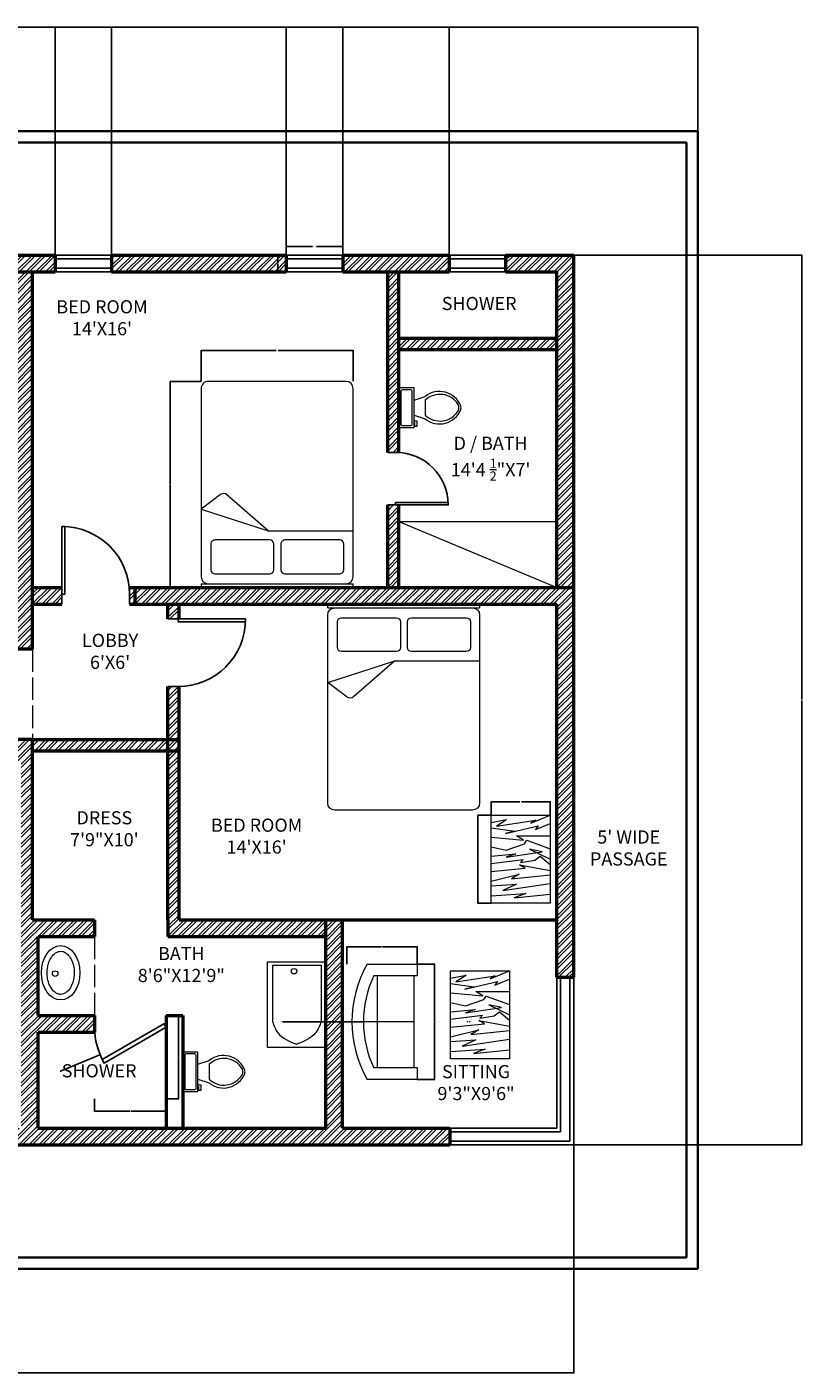
# Model space of a CAD drawing. Units: inches. Extents: x -249 to 953, y -127 to 590.
# Tile 4 of 4: x 540 to 953, y -127 to 590. Entities that reach past the tile are written whole.
import ezdxf

# ---------------------------------------------------------------- set-up
doc = ezdxf.new("R2010")
doc.units = ezdxf.units.IN
doc.header["$MEASUREMENT"] = 0
doc.linetypes.add('ACAD_ISO02W100', pattern=[15, 12, -3])
for name, color, linetype, lineweight in [('A-ANNO-DIMS', 2, 'Continuous', 18), ('A-AREA-IDEN', 2, 'Continuous', 18), ('A-FLOR-CASE', 8, 'Continuous', 18), ('A-FLOR-FIXT-OVHD', 2, 'ACAD_ISO02W100', 13), ('A-FURN', 42, 'Continuous', 18), ('A-GLAZ', 5, 'Continuous', 25), ('A-WALL', 7, 'Continuous', 50), ('A-WALL-OVHD', 7, 'ACAD_ISO02W100', 18), ('A-WALL-PATT', 8, 'Continuous', 13), ('C-PROP', 7, 'Continuous', 35), ('DOOR', 22, 'Continuous', 25), ('L-ANNO-TEXT', 2, 'Continuous', 18), ('WASHROOM', 2, 'Continuous', 18)]:
    doc.layers.add(name, color=color, linetype=linetype, lineweight=lineweight)
doc.styles.get("Standard").update_dxf_attribs({"font": 'arial.ttf'})
doc.dimstyles.get("Standard").update_dxf_attribs({"dimtxt": 0.18, "dimasz": 0.18, "dimexe": 0.18, "dimexo": 0.0625, "dimgap": 0.09, "dimtad": 0, "dimtih": 1, "dimtoh": 1, "dimdec": 4, "dimzin": 0, "dimdsep": 46, "dimtxsty": 'Standard', "dimcen": 0.09, "dimadec": 0, "dimazin": 0, "dimtfac": 1, "dimtdec": 4, "dimtofl": 0, "dimtmove": 0, "dimatfit": 3, "dimfxl": 1, "dimtolj": 1, "dimtzin": 0, "dimarcsym": 0})

# ---------------------------------------------------------------- blocks, each defined once
blk = doc.blocks.new('*U2')
for p, q in [((0, 0), (0, -6)), ((40, 0), (40, -6))]:
    blk.add_line(p, q)
blk.add_lwpolyline([(0, 0), (0, 40), (1.75, 40), (1.75, 0)], close=True)
blk.add_arc((0, 0), 40, 0, 90)
blk = doc.blocks.new('A$C400A1C0B')
for p, q in [((1.5, 2.035), (0, 2.035)), ((0, 2.035), (0, 2)), ((1.5, 2), (0, 2)), ((1.5, 2), (1.5, 2.035)), ((0, 1.93), (0, 0.07)), ((0.673, 1.902), (0.132, 1.902)), ((1.364, 1.902), (0.823, 1.902)), ((1.5, 0.07), (1.5, 1.93)), ((0.092, 1.862), (0.092, 1.607)), ((0.713, 1.607), (0.713, 1.862)), ((0.783, 1.862), (0.783, 1.607)), ((1.404, 1.607), (1.404, 1.862)), ((0.839, 1.476), (0, 1.476)), ((0.132, 1.567), (0.673, 1.567)), ((0.823, 1.567), (1.364, 1.567)), ((1.5, 1.261), (0.839, 1.476)), ((0.839, 1.476), (1.245, 1.12)), ((1.308, 1.117), (1.5, 1.261)), ((0.07, 0), (1.43, 0))]:
    blk.add_line(p, q)
for centre, radius, start, end in [((0.07, 1.93), 0.07, 90, 180), ((1.43, 1.93), 0.07, 0, 90), ((0.132, 1.862), 0.04, 90, 180), ((0.673, 1.862), 0.04, 0, 90), ((0.823, 1.862), 0.04, 90, 180), ((1.364, 1.862), 0.04, 0, 90), ((0.132, 1.607), 0.04, 180, 270), ((0.673, 1.607), 0.04, 270, 0), ((0.823, 1.607), 0.04, 180, 270), ((1.364, 1.607), 0.04, 270, 0), ((1.278, 1.158), 0.05, 228.6958, 306.7579), ((0.07, 0.07), 0.07, 180, 270), ((1.43, 0.07), 0.07, 270, 0)]:
    blk.add_arc(centre, radius, start, end)
blk = doc.blocks.new('A$C01575E38')
for p, q in [((0, 0), (0, 0.65)), ((0, 0), (0, 0.65)), ((0.15, 0), (0.15, 0.563)), ((0.15, 0), (0.15, 0.563)), ((0.75, 0.039), (0.75, 0.7)), ((0.75, 0.039), (0.75, 0.7)), ((1.35, 0), (1.35, 0.563)), ((1.35, 0), (1.35, 0.563)), ((1.5, 0.65), (1.5, 0)), ((1.5, 0.65), (1.5, 0)), ((0.15, 0.515), (1.35, 0.515)), ((0.15, 0.515), (1.35, 0.515)), ((0.15, 0), (0, 0)), ((0.15, 0), (0, 0)), ((0.15, 0.039), (1.35, 0.039)), ((0.15, 0.039), (1.35, 0.039)), ((1.5, 0), (1.35, 0)), ((1.5, 0), (1.35, 0))]:
    blk.add_line(p, q)
for centre, radius, start, end in [((0.75, -0.656), 1.506, 60.1372, 119.8628), ((0.75, -0.656), 1.506, 60.1372, 119.8628), ((0.75, -0.685), 1.385, 64.3208, 115.6792), ((0.75, -0.685), 1.385, 64.3208, 115.6792)]:
    blk.add_arc(centre, radius, start, end)
blk = doc.blocks.new('Door - Imperial')
for p, q in [((0, 0), (0, -5)), ((30, 0), (30, -5))]:
    blk.add_line(p, q)
blk.add_lwpolyline([(0, 0), (25.98, 15), (26.86, 13.48), (0.87, -1.52)], close=True)
blk.add_arc((0, 0), 30, 0, 30)
blk = doc.blocks.new('*U11')
for p, q in [((241, -152), (241, -51)), ((-254, -216), (-203, -216)), ((-254, -241), (-254, -216)), ((-178, -241), (-254, -241)), ((-203, -216), (-203, -203)), ((-178, -203), (-178, -241)), ((-102, -203), (-152, -356)), ((102, -356), (-102, -356)), ((102, -203), (152, -356))]:
    blk.add_line(p, q)
blk.add_lwpolyline([(267, -203), (267, 0), (-267, 0), (-267, -203)], close=True)
for points in [[(-241, -51), (-241, -152)], [(216, -25), (-216, -25)], [(-216, -178), (216, -178)]]:
    blk.add_lwpolyline(points)
for centre, radius, start, end in [((-219, -48), 22.5, 81.8699, 188.1301), ((-219, -156), 22.5, 171.8699, 278.1301), ((219, -48), 22.5, 351.8699, 98.1301), ((219, -156), 22.5, 261.8699, 8.1301), ((89, -548), 309, 141.4691, 247.9714), ((107, -554), 288, 136.3677, 238.9468), ((-89, -548), 309, 292.0284, 38.5307), ((-107, -554), 288, 301.053, 43.6321), ((0, -708), 102, 245.7318, 294.2682), ((0, -737), 102, 254.8605, 285.1395)]:
    blk.add_arc(centre, radius, start, end)
blk = doc.blocks.new('TABLE-OCCASIONAL-GRAIN')
for p, q in [((0, 42.84), (8.23, 44.45)), ((2.86, 40.93), (23.72, 44.22)), ((8.23, 44.45), (6, 42.99)), ((21.04, 42.61), (31.38, 46.82)), ((23.72, 44.22), (21.04, 42.61)), ((0, 40.01), (12.61, 38.25)), ((6, 42.99), (2.86, 40.93)), ((7.55, 37.1), (24.96, 41.05)), ((12.61, 38.25), (7.55, 37.1)), ((23.65, 39.17), (31.38, 42.39)), ((24.96, 41.05), (23.65, 39.17)), ((0, 35.04), (17.13, 33.51)), ((0, 29.97), (0, 29.97)), ((0, 29.97), (7.93, 28.13)), ((7.93, 28.13), (17.75, 31.5)), ((17.13, 33.51), (13.53, 35.8)), ((13.53, 35.8), (31.38, 35.8)), ((17.75, 31.5), (18.89, 33.41)), ((18.89, 33.41), (31.38, 28.82)), ((0, 24.99), (13.07, 26.14)), ((0, 21.15), (7.09, 22)), ((7.09, 22), (17.01, 23.17)), ((8.01, 24.46), (27.17, 27.21)), ((13.07, 26.14), (8.01, 24.46)), ((17.01, 23.17), (15.52, 21.54)), ((15.52, 21.54), (23.18, 22.91)), ((27.17, 27.21), (20.43, 28.67)), ((20.43, 28.67), (31.38, 23.41)), ((23.18, 22.91), (26.02, 24.98)), ((26.02, 24.98), (31.38, 20.54)), ((0, 21.15), (0, 21.15)), ((0, 16.87), (18.13, 18.55)), ((0, 11.74), (14.98, 15.34)), ((14.98, 15.34), (10.84, 12.89)), ((10.84, 12.89), (31.38, 15.11)), ((18.13, 18.55), (15.06, 20.31)), ((15.06, 20.31), (31.38, 17.4)), ((0, 9.2), (13.45, 10.04)), ((6.25, 6.67), (31.38, 10.34)), ((13.45, 10.04), (6.25, 6.67)), ((0, 3.83), (18.43, 5.05)), ((18.43, 5.05), (12.22, 2.76)), ((12.22, 2.76), (31.38, 4.67))]:
    blk.add_line(p, q)
blk.add_lwpolyline([(0, 46.82), (31.38, 46.82), (31.38, 0), (0, 0)], close=True)
blk = doc.blocks.new('WIN-30IN')
for p, q in [((0, 9), (30, 9)), ((0, 7), (30, 7)), ((0, 2), (30, 2)), ((0, 0), (30, 0))]:
    blk.add_line(p, q)
blk = doc.blocks.new('*D33')
at = {"layer": 'A-ANNO-DIMS', "color": 0, "lineweight": -2, "transparency": 16777216}
for p, q in [((632.88, 401.6), (616.31, 401.6)), ((616.49, 401.42), (616.49, 346.95)), ((616.49, 292.11), (616.49, 346.59)), ((632.88, 291.93), (616.31, 291.93))]:
    blk.add_line(p, q, dxfattribs=at)
at = {"layer": 'A-ANNO-DIMS', "color": 0, "transparency": 16777216}
for points in [[(616.46, 401.42), (616.52, 401.42), (616.49, 401.6)], [(616.46, 292.11), (616.52, 292.11), (616.49, 291.93)]]:
    blk.add_solid(points, dxfattribs=at)
at = {"layer": 'Defpoints', "color": 0, "transparency": 16777216}
for p in [(632.94, 401.6), (616.49, 291.93), (632.94, 291.93)]:
    blk.add_point(p, dxfattribs=at)
at = {"layer": 'A-ANNO-DIMS', "color": 0, "transparency": 16777216, "insert": (616.49, 346.77), "char_height": 0.18, "attachment_point": 5}
blk.add_mtext('\\A1;BED 110 TYP.', dxfattribs=at)
blk = doc.blocks.new('*D34')
at = {"layer": 'A-ANNO-DIMS', "color": 0, "lineweight": -2, "transparency": 16777216}
for p, q in [((632.94, 401.67), (632.94, 418.24)), ((633.12, 418.06), (672.83, 418.06)), ((713.6, 418.06), (673.89, 418.06)), ((713.78, 401.67), (713.78, 418.24))]:
    blk.add_line(p, q, dxfattribs=at)
at = {"layer": 'A-ANNO-DIMS', "color": 0, "transparency": 16777216}
for points in [[(633.12, 418.09), (633.12, 418.03), (632.94, 418.06)], [(713.6, 418.09), (713.6, 418.03), (713.78, 418.06)]]:
    blk.add_solid(points, dxfattribs=at)
at = {"layer": 'Defpoints', "color": 0, "transparency": 16777216}
for p in [(632.94, 418.06), (632.94, 401.6), (713.78, 401.6)]:
    blk.add_point(p, dxfattribs=at)
at = {"layer": 'A-ANNO-DIMS', "color": 0, "transparency": 16777216, "insert": (673.36, 418.06), "char_height": 0.18, "attachment_point": 5}
blk.add_mtext('\\A1;81 TYP.', dxfattribs=at)
blk = doc.blocks.new('*D39')
at = {"layer": 'A-ANNO-DIMS', "color": 0, "lineweight": -2, "transparency": 16777216}
for p, q in [((787.21, 170.6), (780.07, 170.6)), ((780.25, 170.42), (780.25, 147.37)), ((780.25, 123.96), (780.25, 147.01)), ((787.21, 123.78), (780.07, 123.78))]:
    blk.add_line(p, q, dxfattribs=at)
at = {"layer": 'A-ANNO-DIMS', "color": 0, "transparency": 16777216}
for points in [[(780.22, 170.42), (780.28, 170.42), (780.25, 170.6)], [(780.22, 123.96), (780.28, 123.96), (780.25, 123.78)]]:
    blk.add_solid(points, dxfattribs=at)
at = {"layer": 'Defpoints', "color": 0, "transparency": 16777216}
for p in [(780.25, 170.6), (787.27, 170.6), (787.27, 123.78)]:
    blk.add_point(p, dxfattribs=at)
at = {"layer": 'A-ANNO-DIMS', "color": 0, "transparency": 16777216, "insert": (780.25, 147.19), "char_height": 0.18, "attachment_point": 5}
blk.add_mtext('\\A1;SIDE TABLE 47 TYP.', dxfattribs=at)
blk = doc.blocks.new('*D40')
at = {"layer": 'A-ANNO-DIMS', "color": 0, "lineweight": -2, "transparency": 16777216}
for p, q in [((787.27, 170.66), (787.27, 177.8)), ((787.45, 177.62), (802.44, 177.62)), ((818.47, 177.62), (803.49, 177.62)), ((818.65, 170.66), (818.65, 177.8))]:
    blk.add_line(p, q, dxfattribs=at)
at = {"layer": 'A-ANNO-DIMS', "color": 0, "transparency": 16777216}
for points in [[(787.45, 177.65), (787.45, 177.59), (787.27, 177.62)], [(818.47, 177.65), (818.47, 177.59), (818.65, 177.62)]]:
    blk.add_solid(points, dxfattribs=at)
at = {"layer": 'Defpoints', "color": 0, "transparency": 16777216}
for p in [(818.65, 177.62), (787.27, 170.6), (818.65, 170.6)]:
    blk.add_point(p, dxfattribs=at)
at = {"layer": 'A-ANNO-DIMS', "color": 0, "transparency": 16777216, "insert": (802.96, 177.62), "char_height": 0.18, "attachment_point": 5}
blk.add_mtext('\\A1;31 TYP.', dxfattribs=at)
blk = doc.blocks.new('*D41')
at = {"layer": 'A-ANNO-DIMS', "color": 0, "lineweight": -2, "transparency": 16777216}
for p, q in [((678.24, 468.99), (678.24, 473.61)), ((678.42, 473.43), (692.12, 473.43)), ((708.06, 473.43), (694.36, 473.43)), ((708.24, 468.99), (708.24, 473.61))]:
    blk.add_line(p, q, dxfattribs=at)
at = {"layer": 'A-ANNO-DIMS', "color": 0, "transparency": 16777216}
for points in [[(678.42, 473.46), (678.42, 473.4), (678.24, 473.43)], [(708.06, 473.46), (708.06, 473.4), (708.24, 473.43)]]:
    blk.add_solid(points, dxfattribs=at)
at = {"layer": 'Defpoints', "color": 0, "transparency": 16777216}
for p in [(708.24, 473.43), (678.24, 468.93), (708.24, 468.93)]:
    blk.add_point(p, dxfattribs=at)
at = {"layer": 'A-ANNO-DIMS', "color": 0, "transparency": 16777216, "insert": (693.24, 473.43), "char_height": 0.18, "attachment_point": 5}
blk.add_mtext('\\A1;WINDOW 30 TYP.', dxfattribs=at)
blk = doc.blocks.new('*D42')
at = {"layer": 'A-ANNO-DIMS', "color": 0, "lineweight": -2, "transparency": 16777216}
for p, q in [((678.18, 468.93), (673.56, 468.93)), ((673.74, 468.75), (673.74, 464.61)), ((678.18, 459.93), (673.56, 459.93)), ((673.74, 460.11), (673.74, 464.25))]:
    blk.add_line(p, q, dxfattribs=at)
at = {"layer": 'A-ANNO-DIMS', "color": 0, "transparency": 16777216}
for points in [[(673.71, 468.75), (673.77, 468.75), (673.74, 468.93)], [(673.71, 460.11), (673.77, 460.11), (673.74, 459.93)]]:
    blk.add_solid(points, dxfattribs=at)
at = {"layer": 'Defpoints', "color": 0, "transparency": 16777216}
for p in [(673.74, 468.93), (678.24, 468.93), (678.24, 459.93)]:
    blk.add_point(p, dxfattribs=at)
at = {"layer": 'A-ANNO-DIMS', "color": 0, "transparency": 16777216, "insert": (673.74, 464.43), "char_height": 0.18, "attachment_point": 5}
blk.add_mtext('\\A1;9 TYP.', dxfattribs=at)
blk = doc.blocks.new('*D47')
at = {"layer": 'A-ANNO-DIMS', "color": 0, "lineweight": -2, "transparency": 16777216}
for p, q in [((747.96, 91.22), (757.28, 91.22)), ((757.1, 91.04), (757.1, 60.73)), ((757.1, 30.06), (757.1, 60.37)), ((747.96, 29.88), (757.28, 29.88))]:
    blk.add_line(p, q, dxfattribs=at)
at = {"layer": 'A-ANNO-DIMS', "color": 0, "transparency": 16777216}
for points in [[(757.07, 91.04), (757.13, 91.04), (757.1, 91.22)], [(757.07, 30.06), (757.13, 30.06), (757.1, 29.88)]]:
    blk.add_solid(points, dxfattribs=at)
at = {"layer": 'Defpoints', "color": 0, "transparency": 16777216}
for p in [(747.9, 91.22), (757.1, 91.22), (747.9, 29.88)]:
    blk.add_point(p, dxfattribs=at)
at = {"layer": 'A-ANNO-DIMS', "color": 0, "transparency": 16777216, "insert": (757.1, 60.55), "char_height": 0.18, "attachment_point": 5}
blk.add_mtext('\\A1;CURVED SOFA 61', dxfattribs=at)
blk = doc.blocks.new('*D48')
at = {"layer": 'A-ANNO-DIMS', "color": 0, "lineweight": -2, "transparency": 16777216}
for p, q in [((710.41, 91.28), (710.41, 100.6)), ((710.59, 100.42), (728.94, 100.42)), ((747.72, 100.42), (729.38, 100.42)), ((747.9, 91.28), (747.9, 100.6))]:
    blk.add_line(p, q, dxfattribs=at)
at = {"layer": 'A-ANNO-DIMS', "color": 0, "transparency": 16777216}
for points in [[(710.59, 100.45), (710.59, 100.39), (710.41, 100.42)], [(747.72, 100.45), (747.72, 100.39), (747.9, 100.42)]]:
    blk.add_solid(points, dxfattribs=at)
at = {"layer": 'Defpoints', "color": 0, "transparency": 16777216}
for p in [(710.41, 100.42), (710.41, 91.22), (747.9, 91.22)]:
    blk.add_point(p, dxfattribs=at)
at = {"layer": 'A-ANNO-DIMS', "color": 0, "transparency": 16777216, "insert": (729.16, 100.42), "char_height": 0.18, "attachment_point": 5}
blk.add_mtext('\\A1;37', dxfattribs=at)
blk = doc.blocks.new('*D49')
at = {"layer": 'A-ANNO-DIMS', "color": 0, "lineweight": -2, "transparency": 16777216}
for p, q in [((614.3, 63.93), (621.07, 63.93)), ((620.89, 63.75), (620.89, 41.93)), ((620.89, 19.75), (620.89, 41.57)), ((614.3, 19.57), (621.07, 19.57))]:
    blk.add_line(p, q, dxfattribs=at)
at = {"layer": 'A-ANNO-DIMS', "color": 0, "transparency": 16777216}
for points in [[(620.86, 63.75), (620.92, 63.75), (620.89, 63.93)], [(620.86, 19.75), (620.92, 19.75), (620.89, 19.57)]]:
    blk.add_solid(points, dxfattribs=at)
at = {"layer": 'Defpoints', "color": 0, "transparency": 16777216}
for p in [(614.24, 63.93), (614.24, 19.57), (620.89, 19.57)]:
    blk.add_point(p, dxfattribs=at)
at = {"layer": 'A-ANNO-DIMS', "color": 0, "transparency": 16777216, "insert": (620.89, 41.75), "char_height": 0.18, "attachment_point": 5}
blk.add_mtext('\\A1;BATH DOOR 44', dxfattribs=at)
blk = doc.blocks.new('*D50')
at = {"layer": 'A-ANNO-DIMS', "color": 0, "lineweight": -2, "transparency": 16777216}
for p, q in [((576.22, 19.51), (576.22, 12.74)), ((614.24, 19.51), (614.24, 12.74)), ((576.4, 12.92), (595.01, 12.92)), ((614.06, 12.92), (595.45, 12.92))]:
    blk.add_line(p, q, dxfattribs=at)
at = {"layer": 'A-ANNO-DIMS', "color": 0, "transparency": 16777216}
for points in [[(576.4, 12.95), (576.4, 12.89), (576.22, 12.92)], [(614.06, 12.95), (614.06, 12.89), (614.24, 12.92)]]:
    blk.add_solid(points, dxfattribs=at)
at = {"layer": 'Defpoints', "color": 0, "transparency": 16777216}
for p in [(576.22, 19.57), (614.24, 19.57), (576.22, 12.92)]:
    blk.add_point(p, dxfattribs=at)
at = {"layer": 'A-ANNO-DIMS', "color": 0, "transparency": 16777216, "insert": (595.23, 12.92), "char_height": 0.18, "attachment_point": 5}
blk.add_mtext('\\A1;38', dxfattribs=at)
blk = doc.blocks.new('*D51')
at = {"layer": 'A-ANNO-DIMS', "color": 0, "lineweight": -2, "transparency": 16777216}
for p, q in [((-193.28, 534.99), (-193.28, 590.41)), ((-193.1, 590.23), (351.51, 590.23)), ((897.04, 590.23), (352.42, 590.23)), ((897.22, 534.99), (897.22, 590.41))]:
    blk.add_line(p, q, dxfattribs=at)
at = {"layer": 'A-ANNO-DIMS', "color": 0, "transparency": 16777216}
for points in [[(-193.1, 590.26), (-193.1, 590.2), (-193.28, 590.23)], [(897.04, 590.26), (897.04, 590.2), (897.22, 590.23)]]:
    blk.add_solid(points, dxfattribs=at)
at = {"layer": 'Defpoints', "color": 0, "transparency": 16777216}
for p in [(897.22, 590.23), (-193.28, 534.93), (897.22, 534.93)]:
    blk.add_point(p, dxfattribs=at)
at = {"layer": 'A-ANNO-DIMS', "color": 0, "transparency": 16777216, "insert": (351.97, 590.23), "char_height": 0.18, "attachment_point": 5}
blk.add_mtext('\\A1;1090.5', dxfattribs=at)
blk = doc.blocks.new('*D53')
at = {"layer": 'A-ANNO-DIMS', "color": 0, "lineweight": -2, "transparency": 16777216}
for p, q in [((1.72, -5.13), (1.72, -126.55)), ((831.22, -5.13), (831.22, -126.55)), ((1.9, -126.37), (416.07, -126.37)), ((831.04, -126.37), (416.86, -126.37))]:
    blk.add_line(p, q, dxfattribs=at)
at = {"layer": 'A-ANNO-DIMS', "color": 0, "transparency": 16777216}
for points in [[(1.9, -126.34), (1.9, -126.4), (1.72, -126.37)], [(831.04, -126.34), (831.04, -126.4), (831.22, -126.37)]]:
    blk.add_solid(points, dxfattribs=at)
at = {"layer": 'Defpoints', "color": 0, "transparency": 16777216}
for p in [(1.72, -5.07), (831.22, -5.07), (831.22, -126.37)]:
    blk.add_point(p, dxfattribs=at)
at = {"layer": 'A-ANNO-DIMS', "color": 0, "transparency": 16777216, "insert": (416.47, -126.37), "char_height": 0.18, "attachment_point": 5}
blk.add_mtext('\\A1;829.5', dxfattribs=at)
blk = doc.blocks.new('*D54')
at = {"layer": 'A-ANNO-DIMS', "color": 0, "lineweight": -2, "transparency": 16777216}
for p, q in [((831.278192, 468.930575), (952.695692, 468.930575)), ((952.515692, 468.750575), (952.515692, 232.110575)), ((952.515692, -4.889425), (952.515692, 231.750575)), ((831.278192, -5.069425), (952.695692, -5.069425))]:
    blk.add_line(p, q, dxfattribs=at)
at = {"layer": 'A-ANNO-DIMS', "color": 0, "transparency": 16777216}
for points in [[(952.485692, 468.750575), (952.545692, 468.750575), (952.515692, 468.930575)], [(952.485692, -4.889425), (952.545692, -4.889425), (952.515692, -5.069425)]]:
    blk.add_solid(points, dxfattribs=at)
at = {"layer": 'Defpoints', "color": 0, "transparency": 16777216}
for p in [(831.215692, 468.930575), (952.515692, 468.930575), (831.215692, -5.069425)]:
    blk.add_point(p, dxfattribs=at)
at = {"layer": 'A-ANNO-DIMS', "color": 0, "transparency": 16777216, "insert": (952.515692, 231.930575), "char_height": 0.18, "attachment_point": 5}
blk.add_mtext('\\A1;474', dxfattribs=at)
blk = doc.blocks.new('*D64')
at = {"layer": 'A-ANNO-DIMS', "color": 0, "lineweight": -2, "transparency": 16777216}
for p, q in [((483.31, 468.99), (483.31, 590.41)), ((483.49, 590.23), (518.89, 590.23)), ((555.08, 590.23), (519.68, 590.23)), ((555.26, 468.99), (555.26, 590.41))]:
    blk.add_line(p, q, dxfattribs=at)
at = {"layer": 'A-ANNO-DIMS', "color": 0, "transparency": 16777216}
for points in [[(483.49, 590.26), (483.49, 590.2), (483.31, 590.23)], [(555.08, 590.26), (555.08, 590.2), (555.26, 590.23)]]:
    blk.add_solid(points, dxfattribs=at)
at = {"layer": 'Defpoints', "color": 0, "transparency": 16777216}
for p in [(555.26, 590.23), (483.31, 468.93), (555.26, 468.93)]:
    blk.add_point(p, dxfattribs=at)
at = {"layer": 'A-ANNO-DIMS', "color": 0, "transparency": 16777216, "insert": (519.28, 590.23), "char_height": 0.18, "attachment_point": 5}
blk.add_mtext('\\A1;71.96', dxfattribs=at)
blk = doc.blocks.new('*D65')
at = {"layer": 'A-ANNO-DIMS', "color": 0, "lineweight": -2, "transparency": 16777216}
for p, q in [((585.26, 468.99), (585.26, 590.41)), ((585.44, 590.23), (631.36, 590.23)), ((678.06, 590.23), (632.15, 590.23)), ((678.24, 468.99), (678.24, 590.41))]:
    blk.add_line(p, q, dxfattribs=at)
at = {"layer": 'A-ANNO-DIMS', "color": 0, "transparency": 16777216}
for points in [[(585.44, 590.26), (585.44, 590.2), (585.26, 590.23)], [(678.06, 590.26), (678.06, 590.2), (678.24, 590.23)]]:
    blk.add_solid(points, dxfattribs=at)
at = {"layer": 'Defpoints', "color": 0, "transparency": 16777216}
for p in [(678.24, 590.23), (585.26, 468.93), (678.24, 468.93)]:
    blk.add_point(p, dxfattribs=at)
at = {"layer": 'A-ANNO-DIMS', "color": 0, "transparency": 16777216, "insert": (631.75, 590.23), "char_height": 0.18, "attachment_point": 5}
blk.add_mtext('\\A1;92.98', dxfattribs=at)
blk = doc.blocks.new('*D66')
at = {"layer": 'A-ANNO-DIMS', "color": 0, "lineweight": -2, "transparency": 16777216}
for p, q in [((708.24, 468.99), (708.24, 590.41)), ((708.42, 590.23), (736.19, 590.23)), ((764.75, 590.23), (736.98, 590.23)), ((764.93, 468.99), (764.93, 590.41))]:
    blk.add_line(p, q, dxfattribs=at)
at = {"layer": 'A-ANNO-DIMS', "color": 0, "transparency": 16777216}
for points in [[(708.42, 590.26), (708.42, 590.2), (708.24, 590.23)], [(764.75, 590.26), (764.75, 590.2), (764.93, 590.23)]]:
    blk.add_solid(points, dxfattribs=at)
at = {"layer": 'Defpoints', "color": 0, "transparency": 16777216}
for p in [(764.93, 590.23), (708.24, 468.93), (764.93, 468.93)]:
    blk.add_point(p, dxfattribs=at)
at = {"layer": 'A-ANNO-DIMS', "color": 0, "transparency": 16777216, "insert": (736.59, 590.23), "char_height": 0.18, "attachment_point": 5}
blk.add_mtext('\\A1;56.69', dxfattribs=at)
blk = doc.blocks.new('*D68')
at = {"layer": 'A-ANNO-DIMS', "color": 0, "lineweight": -2, "transparency": 16777216}
for p, q in [((676.18, 60.55), (712.96, 60.55)), ((774.65, 60.55), (774.83, 60.55)), ((774.74, 60.46), (774.74, 60.64))]:
    blk.add_line(p, q, dxfattribs=at)
at = {"layer": 'A-ANNO-DIMS', "color": 0, "transparency": 16777216}
blk.add_solid([(712.96, 60.58), (712.96, 60.52), (713.14, 60.55)], dxfattribs=at)
at = {"layer": 'Defpoints', "color": 0, "transparency": 16777216}
for p in [(713.14, 60.55), (774.74, 60.55)]:
    blk.add_point(p, dxfattribs=at)
at = {"layer": 'A-ANNO-DIMS', "color": 0, "transparency": 16777216, "insert": (675.57, 60.55), "char_height": 0.18, "attachment_point": 5}
blk.add_mtext('\\A1;2X R61.6', dxfattribs=at)
blk = doc.blocks.new('*D69')
at = {"layer": 'A-ANNO-DIMS', "color": 0, "lineweight": -2, "transparency": 16777216}
for p, q in [((685.3, 60.55), (719.09, 60.55)), ((775.81, 60.55), (775.99, 60.55)), ((775.9, 60.46), (775.9, 60.64))]:
    blk.add_line(p, q, dxfattribs=at)
at = {"layer": 'A-ANNO-DIMS', "color": 0, "transparency": 16777216}
blk.add_solid([(719.09, 60.58), (719.09, 60.52), (719.27, 60.55)], dxfattribs=at)
at = {"layer": 'Defpoints', "color": 0, "transparency": 16777216}
for p in [(719.27, 60.55), (775.9, 60.55)]:
    blk.add_point(p, dxfattribs=at)
at = {"layer": 'A-ANNO-DIMS', "color": 0, "transparency": 16777216, "insert": (684.62, 60.55), "char_height": 0.18, "attachment_point": 5}
blk.add_mtext('\\A1;2X R56.63', dxfattribs=at)
blk = doc.blocks.new('*D70')
at = {"layer": 'A-ANNO-DIMS', "color": 0, "lineweight": -2, "transparency": 16777216}
for p, q in [((614.15, 57.59), (614.33, 57.59)), ((614.24, 57.5), (614.24, 57.68)), ((558.03, 34.31), (578.94, 42.97)), ((557.85, 34.31), (558.03, 34.31))]:
    blk.add_line(p, q, dxfattribs=at)
at = {"layer": 'A-ANNO-DIMS', "color": 0, "transparency": 16777216}
blk.add_solid([(578.93, 43), (578.96, 42.95), (579.11, 43.04)], dxfattribs=at)
at = {"layer": 'Defpoints', "color": 0, "transparency": 16777216}
for p in [(614.24, 57.59), (579.11, 43.04)]:
    blk.add_point(p, dxfattribs=at)
at = {"layer": 'A-ANNO-DIMS', "color": 0, "transparency": 16777216, "insert": (557.18, 34.31), "char_height": 0.18, "attachment_point": 5}
blk.add_mtext('\\A1;4X R38.02', dxfattribs=at)

msp = doc.modelspace()

# ---------------------------------------------------------------- hatches: boundary and pattern name
at = {"layer": 'A-WALL-PATT'}
h = msp.add_hatch(dxfattribs=at)
h.set_pattern_fill('ANSI32', color=256, scale=10)
h.paths.add_polyline_path([(678.2396, 468.9306), (585.2636, 468.9306), (585.2636, 459.9306), (678.2396, 459.9306)])
h.paths.add_polyline_path([(555.2636, 468.9306), (534.2157, 468.9306), (534.2157, 459.9306), (555.2636, 459.9306)])
h.paths.add_polyline_path([(534.2157, 468.9306), (483.3054, 468.9306), (483.3054, 459.9306), (534.2157, 459.9306)])
h.paths.add_polyline_path([(543.2157, 459.9306), (534.2157, 459.9306), (534.2157, 258.9306), (543.2157, 258.9306)])
h = msp.add_hatch(dxfattribs=at)
h.set_pattern_fill('ANSI32', color=256, scale=10)
h.paths.add_polyline_path([(831.2157, 468.9306), (794.9311, 468.9306), (794.9311, 459.9306), (822.2157, 459.9306), (822.2157, 291.9306), (831.2157, 291.9306)])
h.paths.add_polyline_path([(738.2157, 335.8354), (736.4157, 335.8354), (732.2157, 335.8354), (732.2157, 291.9306), (738.2157, 291.9306)])
h.paths.add_polyline_path([(738.2157, 459.9306), (732.2157, 459.9306), (732.2157, 363.8354), (736.4157, 363.8354, -0.01608391), (738.2157, 363.7774)])
h.paths.add_polyline_path([(764.9311, 468.9306), (708.2396, 468.9306), (708.2396, 459.9306), (764.9311, 459.9306)])
h = msp.add_hatch(dxfattribs=at)
h.set_pattern_fill('ANSI32', color=256, scale=10)
h.paths.add_polyline_path([(738.2157, 424.5675), (738.2157, 418.5675), (822.2157, 418.5675), (822.2157, 424.5675)])
h = msp.add_hatch(dxfattribs=at)
h.set_pattern_fill('ANSI32', color=256, scale=10)
h.paths.add_polyline_path([(831.2157, 291.9306), (597.6638, 291.9306), (597.6638, 282.9306), (822.2157, 282.9306), (822.2157, 84.246), (831.2157, 84.246)])
h.paths.add_polyline_path([(597.6638, 291.9306), (594.6732, 291.9306, -0.02504709), (594.8536, 288.3306), (594.8536, 282.9306), (597.6638, 282.9306)])
h.paths.add_polyline_path([(558.8536, 288.3306), (558.8536, 291.9306), (543.2157, 291.9306), (543.2157, 282.9306), (558.8536, 282.9306)])
h = msp.add_hatch(dxfattribs=at)
h.set_pattern_fill('ANSI32', color=256, scale=10)
h.paths.add_polyline_path([(621.2157, 282.9306), (615.2157, 282.9306), (615.2157, 275.0875), (620.6157, 275.0875), (621.2157, 275.0875)])
h.paths.add_polyline_path([(621.2157, 239.0925, -0.00416688), (620.6157, 239.0875), (615.2157, 239.0875), (615.2157, 210.9306), (621.2157, 210.9306)])
h.paths.add_polyline_path([(615.2157, 210.9306), (543.2157, 210.9306), (543.2157, 204.9306), (615.2157, 204.9306)])
h.paths.add_polyline_path([(621.2157, 210.9306), (615.2157, 210.9306), (615.2157, 204.9306), (621.2157, 204.9306)])
h.paths.add_polyline_path([(621.2157, 204.9306), (615.2157, 204.9306), (615.2157, 114.9306), (615.2157, 105.9306), (699.2157, 105.9306), (699.2157, 114.9306), (621.2157, 114.9306)])
h = msp.add_hatch(dxfattribs=at)
h.set_pattern_fill('ANSI32', color=256, scale=10)
h.paths.add_polyline_path([(765.2157, 3.9306), (708.2157, 3.9306), (708.2157, 114.9306), (699.2157, 114.9306), (699.2157, 3.9306), (546.2157, 3.9306), (546.2157, 54.9306), (576.2157, 54.9306), (576.2157, 63.9306), (546.2157, 63.9306), (546.2157, 105.9306), (576.2157, 105.9306), (576.2157, 114.9306), (543.2157, 114.9306), (543.2157, 210.9306), (534.2157, 210.9306), (534.2157, 207.9306), (508.5171, 207.9306), (508.5171, 198.9306), (537.2157, 198.9306), (537.2157, 3.9306), (417.2157, 3.9306), (417.2157, 207.9306), (411.2157, 207.9306), (411.2157, 3.9306), (369.1469, 3.9306, -0.05252224), (369.6736, -1.0697), (369.6736, -5.0694), (765.2157, -5.0694)])

# ---------------------------------------------------------------- linework, layer by layer
at = {"layer": 'A-FLOR-CASE'}
for q in [(822.2157, 326.9113), (822.2157, 291.9306)]:
    msp.add_line((738.2157, 326.9113), q, dxfattribs=at)
at = {"layer": 'A-FLOR-FIXT-OVHD'}
msp.add_line((576.2157, 105.9306), (576.2157, 63.9306), dxfattribs=at)
at = {"layer": 'A-GLAZ'}
for p, q in [((822.2157, 84.246), (822.2157, 3.9306)), ((824.2157, 84.246), (824.2157, 1.9306)), ((829.2157, 84.246), (829.2157, -3.0694)), ((831.2157, 84.246), (831.2157, -5.0694)), ((765.2157, 3.9306), (822.2157, 3.9306)), ((765.2157, 1.9306), (824.2157, 1.9306)), ((765.2157, -3.0694), (829.2157, -3.0694)), ((765.2157, -5.0694), (831.2157, -5.0694))]:
    msp.add_line(p, q, dxfattribs=at)
at = {"layer": 'A-WALL'}
for p, q in [((483.3054, 468.9306), (555.2636, 468.9306)), ((555.2636, 468.9306), (555.2636, 459.9306)), ((585.2636, 468.9306), (585.2636, 459.9306)), ((585.2636, 468.9306), (678.2396, 468.9306)), ((678.2396, 468.9306), (678.2396, 459.9306)), ((708.2396, 468.9306), (708.2396, 459.9306)), ((708.2396, 468.9306), (764.9311, 468.9306)), ((764.9311, 468.9306), (764.9311, 459.9306)), ((794.9311, 468.9306), (794.9311, 459.9306)), ((794.9311, 468.9306), (831.2157, 468.9306)), ((831.2157, 84.246), (831.2157, 468.9306)), ((483.3054, 459.9306), (555.2636, 459.9306)), ((543.2157, 258.9306), (543.2157, 459.9306)), ((585.2636, 459.9306), (678.2396, 459.9306)), ((708.2396, 459.9306), (764.9311, 459.9306)), ((732.2157, 363.8354), (732.2157, 459.9306)), ((738.2157, 363.7774), (738.2157, 459.9306)), ((794.9311, 459.9306), (822.2157, 459.9306)), ((822.2157, 291.9306), (822.2157, 459.9306)), ((738.2157, 424.5675), (822.2157, 424.5675)), ((738.2157, 418.5675), (822.2157, 418.5675)), ((732.2157, 291.9306), (732.2157, 335.8354)), ((738.2157, 291.9306), (738.2157, 335.8354)), ((543.2157, 291.9306), (558.8536, 291.9306)), ((594.6732, 291.9306), (831.2157, 291.9306)), ((597.6638, 291.9306), (597.6638, 282.9306)), ((543.2157, 282.9306), (558.8536, 282.9306)), ((594.8536, 282.9306), (822.2157, 282.9306)), ((615.2157, 275.0875), (615.2157, 282.9306)), ((621.2157, 275.0875), (621.2157, 282.9306)), ((822.2157, 84.246), (822.2157, 282.9306)), ((543.2157, 258.9306), (534.2157, 258.9306)), ((615.2157, 114.9306), (615.2157, 239.0875)), ((621.2157, 114.9306), (621.2157, 239.0925)), ((543.2157, 210.9306), (534.2157, 210.9306)), ((543.2157, 210.9306), (621.2157, 210.9306)), ((543.2157, 114.9306), (543.2157, 210.9306)), ((543.2157, 204.9306), (621.2157, 204.9306)), ((543.2157, 114.9306), (576.2157, 114.9306)), ((576.2157, 114.9306), (576.2157, 105.9306)), ((615.2157, 114.9306), (615.2157, 105.9306)), ((621.2157, 114.9306), (822.2157, 114.9306)), ((699.2157, 3.9306), (699.2157, 114.9306)), ((708.2157, 3.9306), (708.2157, 114.9306)), ((546.2157, 105.9306), (576.2157, 105.9306)), ((546.2157, 63.9306), (546.2157, 105.9306)), ((615.2157, 105.9306), (699.2157, 105.9306)), ((822.2157, 84.246), (831.2157, 84.246)), ((546.2157, 63.9306), (576.2157, 63.9306)), ((576.2157, 63.9306), (576.2157, 54.9306)), ((614.238, 63.9306), (614.238, 3.9306)), ((614.238, 63.9306), (623.238, 63.9306)), ((623.238, 63.9306), (623.238, 3.9306)), ((546.2157, 3.9306), (546.2157, 54.9306)), ((546.2157, 54.9306), (576.2157, 54.9306)), ((546.2157, 3.9306), (699.2157, 3.9306)), ((708.2157, 3.9306), (765.2157, 3.9306)), ((765.2157, 3.9306), (765.2157, -5.0694)), ((369.6736, -5.0694), (765.2157, -5.0694))]:
    msp.add_line(p, q, dxfattribs=at)
at = {"layer": 'A-WALL-OVHD'}
msp.add_line((543.2157, 258.9306), (543.2157, 210.9306), dxfattribs=at)
at = {"layer": 'C-PROP'}
for p, q in [((-193.2843, 534.9306), (897.2157, 534.9306)), ((897.2157, -71.0694), (897.2157, 534.9306)), ((-187.2843, 528.9306), (891.2157, 528.9306)), ((891.2157, -65.0694), (891.2157, 528.9306)), ((-193.2843, -71.0694), (897.2157, -71.0694)), ((-187.2843, -65.0694), (891.2157, -65.0694))]:
    msp.add_line(p, q, dxfattribs=at)
at = {"layer": 'WASHROOM'}
for p, q in [((670.9014, 90.6457), (670.9014, 60.6255)), ((670.9014, 90.6457), (696.8212, 90.6457)), ((696.8212, 90.6457), (696.8212, 60.6255))]:
    msp.add_line(p, q, dxfattribs=at)
msp.add_lwpolyline([(668.298, 92.5389), (699.2157, 92.5389), (699.2157, 46.7714), (668.298, 46.7714)], close=True, dxfattribs=at)
for centre, radius in [((555.2616, 86.2056), 1.477), ((682.3597, 87.4762), 1.4562)]:
    msp.add_circle(centre, radius, dxfattribs=at)
msp.add_ellipse((558.1591, 86.637), major_axis=(0, -14.4848), ratio=0.70563009, dxfattribs=at)
for points, knots in [([(558.1591, 75.1522), (558.6444, 75.1522), (559.1311, 75.2343), (560.1282, 75.5859), (560.6388, 75.8576), (561.6546, 76.6214), (562.1584, 77.1141), (563.1004, 78.313), (563.538, 79.0187), (564.2935, 80.6003), (564.6114, 81.4757), (565.0917, 83.3329), (565.254, 84.3145), (565.4332, 86.6721), (565.3751, 88.0619), (564.9473, 90.7137), (564.5775, 91.9746), (563.6006, 94.198), (562.9942, 95.1585), (561.8115, 96.5188), (561.2559, 96.9932), (560.1517, 97.6864), (559.605, 97.9069), (558.5384, 98.1388), (558.0162, 98.1529), (556.9551, 97.983), (556.4133, 97.7966), (555.3115, 97.1778), (554.7532, 96.7433), (553.6866, 95.6129), (553.1798, 94.9174), (552.2912, 93.3078), (551.9098, 92.3945), (551.324, 90.4261), (551.1197, 89.3716), (550.9138, 87.2131), (550.9123, 86.1095), (551.1122, 83.9497), (551.3136, 82.8937), (551.8942, 80.9212), (552.2734, 80.0052), (553.1583, 78.3893), (553.6637, 77.6901), (554.7288, 76.5521), (555.2869, 76.1137), (556.389, 75.4876), (556.9313, 75.2979), (557.6955, 75.1712), (557.9273, 75.1522), (558.1591, 75.1522)], [0, 0, 0, 0, 0.24391177, 0.24391177, 0.48782354, 0.48782354, 0.7317353, 0.7317353, 0.97564707, 0.97564707, 1.21955884, 1.21955884, 1.46347061, 1.46347061, 1.7955826, 1.7955826, 2.12769459, 2.12769459, 2.45980658, 2.45980658, 2.72458551, 2.72458551, 2.98936443, 2.98936443, 3.25414336, 3.25414336, 3.51892229, 3.51892229, 3.78370122, 3.78370122, 4.04848015, 4.04848015, 4.31325908, 4.31325908, 4.57803801, 4.57803801, 4.84281693, 4.84281693, 5.10759586, 5.10759586, 5.37237479, 5.37237479, 5.63715372, 5.63715372, 5.90193265, 5.90193265, 6.16671158, 6.16671158, 6.28318531, 6.28318531, 6.28318531, 6.28318531]), ([(670.9014, 60.6255), (671.6637, 58.4794), (673.7829, 52.5129), (679.8634, 50.1101), (683.7569, 48.5715)], [0, 0, 0, 0, 6.59996646, 18.34979425, 18.34979425, 18.34979425, 18.34979425]), ([(696.8212, 60.6255), (695.9829, 58.4809), (693.6727, 52.5707), (687.6159, 50.1279), (683.7569, 48.5715)], [0, 0, 0, 0, 6.69126177, 18.44108956, 18.44108956, 18.44108956, 18.44108956])]:
    msp.add_open_spline(points, degree=3, knots=knots, dxfattribs=at)

# ---------------------------------------------------------------- block references
at = {"layer": 'A-FURN'}
for name, p, xscale, yscale, zscale, rotation in [('A$C400A1C0B', (713.7806, 401.6044), 53.89375545965505, 53.89375545965505, 53.89375545965505, 180), ('A$C01575E38', (747.9015, 29.8754), 40.89768381262322, 40.89768381262322, 40.89768381262322, 90)]:
    msp.add_blockref(name, p, dxfattribs=dict(at, xscale=xscale, yscale=yscale, zscale=zscale, rotation=rotation))
at = {"layer": 'A-FURN', "xscale": -53.89375545965505, "yscale": 53.89375545965505, "zscale": 53.89375545965505}
msp.add_blockref('A$C400A1C0B', (781.1406, 173.2568), dxfattribs=at)
at = {"layer": 'A-FURN'}
for p in [(787.2744, 123.7803), (765.654, 40.866)]:
    msp.add_blockref('TABLE-OCCASIONAL-GRAIN', p, dxfattribs=at)
at = {"layer": 'A-GLAZ'}
for p in [(555.2633, 459.931), (678.2394, 459.931), (764.9309, 459.931)]:
    msp.add_blockref('WIN-30IN', p, dxfattribs=at)
at = {"layer": 'DOOR'}
for name, p, xscale, yscale, zscale, rotation in [('*U2', (736.4157, 335.8354), -0.7000000000000001, 0.7000000000000001, 0.7000000000000001, 270), ('*U2', (620.6157, 275.0875), 0.9, 0.9, 0.9, 270), ('Door - Imperial', (614.238, 57.5935), 1.267411112965237, 1.267411112965237, 1.267411112965237, 180)]:
    msp.add_blockref(name, p, dxfattribs=dict(at, xscale=xscale, yscale=yscale, zscale=zscale, rotation=rotation))
at = {"layer": 'DOOR', "xscale": 0.9, "yscale": 0.9, "zscale": 0.9}
msp.add_blockref('*U2', (558.8536, 288.3306), dxfattribs=at)
at = {"layer": 'WASHROOM', "xscale": 0.0393700787401575, "yscale": 0.0393700787401575, "zscale": 0.0393700787401575, "rotation": 90}
for p in [(738.2157, 387.6044), (623.238, 33.9306)]:
    msp.add_blockref('*U11', p, dxfattribs=at)

# ---------------------------------------------------------------- texts
at = {"layer": 'A-AREA-IDEN', "char_height": 7, "attachment_point": 1}
for s, insert in [("\\A1;\\pxqc;BED ROOM\\P14'X16'", (540.3491, 444.8581)), ('\\A1;\\pxqc;SHOWER', (741.0728, 446.6056)), ('\\A1;\\pxqc;D / BATH\\P14\'4 {\\H0.7x;\\S1/2;}"X7\'', (747.1652, 372.165)), ("\\A1;\\pxqc;LOBBY\\P6'X6'", (544.6574, 267.185)), ('\\A1;\\pxqc;DRESS\\P7\'9"X10\'', (541.6058, 172.7061)), ("\\A1;\\pxqc;BED ROOM\\P14'X16'", (622.6483, 168.7687)), ('\\A1;\\pxqc;BATH\\P8\'6"X12\'9"', (582.575, 100.38)), ('\\A1;\\pxqc;SHOWER', (538.8232, 37.9569)), ('\\A1;\\pxqc;SITTING\\P9\'3"X9\'6"', (739.4064, 37.5013))]:
    msp.add_mtext_dynamic_manual_height_columns(s, width=79.609867, gutter_width=1, heights=[0], dxfattribs=dict(at, insert=insert))
at = {"layer": 'L-ANNO-TEXT', "insert": (820.6926, 162.4361), "char_height": 7, "attachment_point": 1}
msp.add_mtext_dynamic_manual_height_columns("\\A1;\\pxqc;5' WIDE\\PPASSAGE", width=79.609867, gutter_width=1, heights=[0], dxfattribs=at)

# ---------------------------------------------------------------- dimensions: what is measured, and where the dimension line sits
at = {"layer": 'A-ANNO-DIMS'}
for base, p1, p2, override, picture, middle in [((897.2157, 590.2306), (-193.2843, 534.9306), (897.2157, 534.9306), {"dimdec": 1, "dimlfac": 1, "dimrnd": 0, "dimzin": 0, "dimdsep": 46, "dimlunit": 2}, '*D51', (351.9657, 590.2306)), ((555.2636, 590.2306), (483.3054, 468.9306), (555.2636, 468.9306), {"dimdec": 2, "dimlfac": 1, "dimrnd": 0, "dimzin": 0, "dimdsep": 46, "dimlunit": 2}, '*D64', (519.2845, 590.2306)), ((678.2396, 590.2306), (585.2636, 468.9306), (678.2396, 468.9306), {"dimdec": 2, "dimlfac": 1, "dimrnd": 0, "dimzin": 0, "dimdsep": 46, "dimlunit": 2}, '*D65', (631.7516, 590.2306)), ((764.9311, 590.2306), (708.2396, 468.9306), (764.9311, 468.9306), {"dimdec": 2, "dimlfac": 1, "dimrnd": 0, "dimzin": 0, "dimdsep": 46, "dimlunit": 2}, '*D66', (736.5854, 590.2306)), ((831.2157, -126.3694), (1.7157, -5.0694), (831.2157, -5.0694), {"dimdec": 1, "dimlfac": 1, "dimrnd": 0, "dimzin": 0, "dimdsep": 46, "dimlunit": 2}, '*D53', (416.4657, -126.3694))]:
    dim = msp.add_linear_dim(base=base, p1=p1, p2=p2, dimstyle='Standard', override=override, dxfattribs=at)
    dim.commit()
    dim.dimension.update_dxf_attribs({"geometry": picture, "text_midpoint": middle})
for base, p1, p2, text, picture, middle in [((708.2396, 473.4306), (678.2396, 468.9306), (708.2396, 468.9306), 'WINDOW <> TYP.', '*D41', (693.2396, 473.4306)), ((818.6536, 177.6204), (787.2743, 170.5977), (818.6536, 170.5977), '<> TYP.', '*D40', (802.9639, 177.6204))]:
    dim = msp.add_linear_dim(base=base, p1=p1, p2=p2, text=text, dimstyle='Standard', override={"dimdec": 0, "dimlfac": 1, "dimrnd": 0, "dimzin": 0, "dimdsep": 46, "dimlunit": 2}, dxfattribs=at)
    dim.commit()
    dim.dimension.update_dxf_attribs({"geometry": picture, "text_midpoint": middle})
for base, p1, p2, angle, text, picture, middle in [((673.7396, 468.9306), (678.2396, 459.9306), (678.2396, 468.9306), 90, '<> TYP.', '*D42', (673.7396, 464.4306)), ((632.94, 418.0554), (713.7806, 401.6044), (632.94, 401.6044), 180, '<> TYP.', '*D34', (673.3603, 418.0554)), ((616.4889, 291.9306), (632.94, 401.6044), (632.94, 291.9306), 270, 'BED <> TYP.', '*D33', (616.4889, 346.7675)), ((780.2517, 170.5977), (787.2743, 123.7802), (787.2743, 170.5977), 90, 'SIDE TABLE <> TYP.', '*D39', (780.2517, 147.189)), ((757.1035, 91.2219), (747.9015, 29.8754), (747.9015, 91.2219), 90, 'CURVED SOFA <>', '*D47', (757.1035, 60.5487)), ((620.8919, 19.5712), (614.238, 63.9306), (614.238, 19.5712), 270, 'BATH DOOR <>', '*D49', (620.8919, 41.7509))]:
    dim = msp.add_linear_dim(base=base, p1=p1, p2=p2, angle=angle, text=text, dimstyle='Standard', override={"dimdec": 0, "dimlfac": 1, "dimrnd": 0, "dimzin": 0, "dimdsep": 46, "dimlunit": 2}, dxfattribs=at)
    dim.commit()
    dim.dimension.update_dxf_attribs({"geometry": picture, "text_midpoint": middle})
for base, p1, p2, angle, picture, middle in [((952.5157, 468.9306), (831.2157, -5.0694), (831.2157, 468.9306), 90, '*D54', (952.5157, 231.9306)), ((710.412, 100.4239), (747.9015, 91.2219), (710.412, 91.2219), 180, '*D48', (729.1567, 100.4239)), ((576.2157, 12.9173), (614.238, 19.5712), (576.2157, 19.5712), 180, '*D50', (595.2269, 12.9173))]:
    dim = msp.add_linear_dim(base=base, p1=p1, p2=p2, angle=angle, dimstyle='Standard', override={"dimdec": 0, "dimlfac": 1, "dimrnd": 0, "dimzin": 0, "dimdsep": 46, "dimlunit": 2}, dxfattribs=at)
    dim.commit()
    dim.dimension.update_dxf_attribs({"geometry": picture, "text_midpoint": middle})
for center, mpoint, text, override, picture, middle in [((614.238, 57.5935), (579.11, 43.043), '4X <>', {"dimdec": 2, "dimlfac": 1, "dimrnd": 0, "dimzin": 0, "dimdsep": 46, "dimlunit": 2}, '*D70', (557.1772, 34.3127)), ((774.7406, 60.5486), (713.1385, 60.549), '2X <>', {"dimdec": 1, "dimlfac": 1, "dimrnd": 0, "dimzin": 0, "dimdsep": 46, "dimlunit": 2}, '*D68', (676.1772, 60.5492)), ((775.9005, 60.5486), (719.2731, 60.549), '2X <>', {"dimdec": 2, "dimlfac": 1, "dimrnd": 0, "dimzin": 0, "dimdsep": 46, "dimlunit": 2}, '*D69', (685.2966, 60.5492))]:
    dim = msp.add_radius_dim(center=center, mpoint=mpoint, text=text, dimstyle='Standard', override=override, dxfattribs=at)
    dim.commit()
    dim.dimension.update_dxf_attribs({"geometry": picture, "text_midpoint": middle, "dimtype": 164})

doc.saveas('drawing.dxf')
